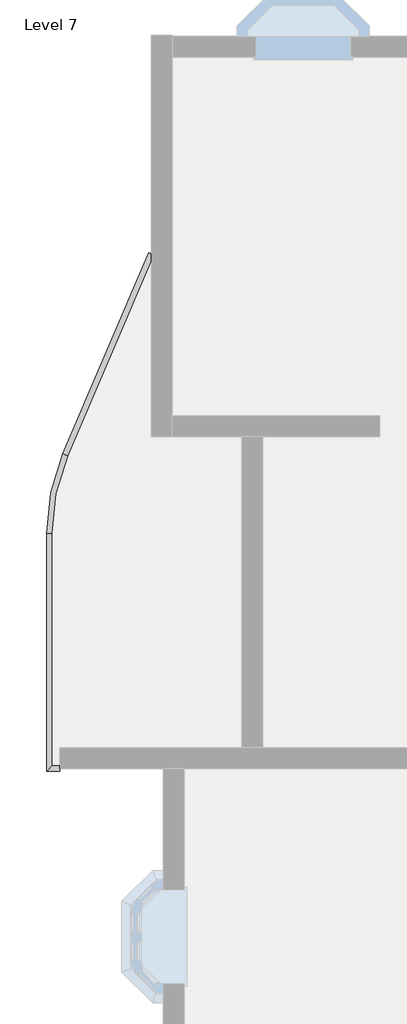
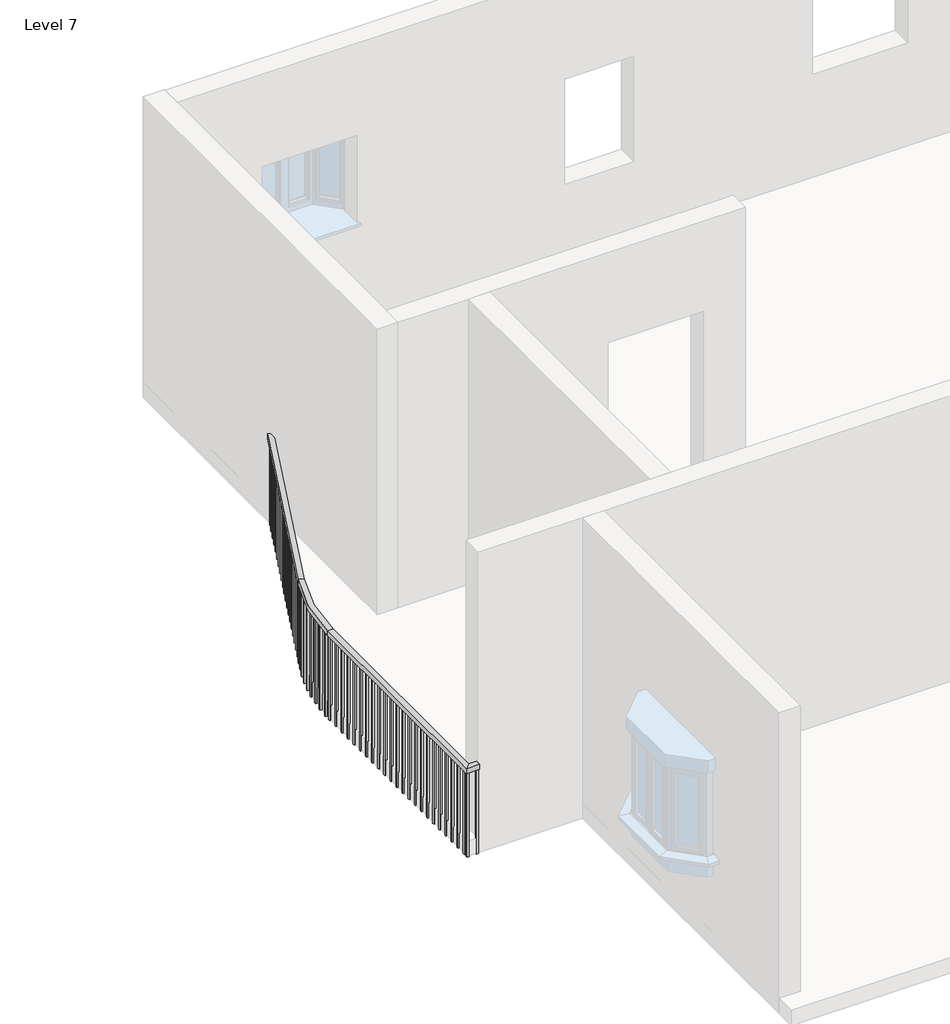
# One storey, part 7 of 14: 1 railing.
"""IFC4 building model written with IfcOpenShell, lengths in millimetres."""

from ifc_helpers import new_model, si_unit, frame, origin, place, context, project, spatial, polyline, circle_curve, outline, extrude, element, save
from ifc_brep_helpers import plane_surface, cylinder_surface, revolved_surface, advanced_brep

model = new_model("IFC4")

# Units and contexts
model_context = context("Model", 3, world=origin())
ifc_project = project(units=[si_unit("LENGTHUNIT", "METRE", prefix="MILLI")], contexts=[model_context])

# Site, building, storey
site = spatial("IfcSite", under=ifc_project)
building = spatial("IfcBuilding", under=site)
storey = spatial("IfcBuildingStorey", under=building, Name="Level 7", Elevation=18288.0)

# Railing
placement = place(None, origin())
element("IfcRailing", 1, ObjectType="Handrail - Rectangular", at=placement, inside=storey, context=model_context, shape_type="SolidModel", body=[
    advanced_brep(
    [(-12381.4379579, -2441.2590879, 19202.4), (-12381.4379579, -2441.2590879, 19151.6), (-12428.1364721, -2421.2618688, 19151.6), (-12428.1364721, -2421.2618688, 19202.4), (-13216.1814979, -4390.5942894, 19202.4), (-13216.1814979, -4390.5942894, 19151.6), (-13262.8800121, -4370.5970703, 19151.6), (-13262.8800121, -4370.5970703, 19202.4), (-13369.987215, -5140.4900045, 19151.6), (-13369.987215, -5140.4900045, 19202.4), (-13420.787215, -5140.4900045, 19151.6), (-13420.787215, -5140.4900045, 19202.4), (-13369.987215, -7396.5416506, 19202.4), (-13369.987215, -7396.5416506, 19151.6), (-13420.787215, -7447.3416506, 19151.6), (-13420.787215, -7447.3416506, 19202.4), (-13293.787215, -7396.5416506, 19202.4), (-13293.787215, -7447.3416506, 19202.4), (-13293.787215, -7447.3416506, 19151.6), (-13293.787215, -7396.5416506, 19151.6)],
    [
        (0, 1),
        (1, 2),
        (2, 3),
        (3, 0),
        (0, 4),
        (4, 5),
        (5, 1),
        (5, 6),
        (6, 2),
        (6, 7),
        (7, 3),
        (7, 4),
        (8, 5, circle_curve(frame((-11464.987215, -5140.4900045, 19151.6), z_axis=(0.0, 0.0, -1.0), x_axis=(-0.9192620907623801, 0.39364604467361003, 0.0)), 1905.0)),
        (4, 9, circle_curve(frame((-11464.987215, -5140.4900045, 19202.4), z_axis=(0.0, 0.0, 1.0), x_axis=(-0.9192620907623801, 0.39364604467361003, 0.0)), 1905.0)),
        (9, 8),
        (10, 6, circle_curve(frame((-11464.987215, -5140.4900045, 19151.6), z_axis=(0.0, 0.0, -1.0), x_axis=(-0.9192620907623801, 0.39364604467361003, 0.0)), 1955.8)),
        (8, 10),
        (11, 7, circle_curve(frame((-11464.987215, -5140.4900045, 19202.4), z_axis=(0.0, 0.0, -1.0), x_axis=(-0.9192620907623801, 0.39364604467361003, 0.0)), 1955.8)),
        (10, 11),
        (11, 9),
        (9, 12),
        (12, 13),
        (13, 8),
        (13, 14),
        (14, 10),
        (14, 15),
        (15, 11),
        (15, 12),
        (16, 17),
        (17, 18),
        (18, 19),
        (19, 16),
        (12, 16),
        (19, 13),
        (18, 14),
        (17, 15),
    ],
    [
        plane_surface(frame((-12404.787215, -2431.2604783, 19202.4), z_axis=(0.39364604467361003, 0.9192620907623801, 0.0), x_axis=(0.9192620907623801, -0.39364604467361003, 0.0))),
        plane_surface(frame((-12381.4379579, -2441.2590879, 19202.4), z_axis=(0.91926209076238, -0.39364604467361014, 0.0), x_axis=(-0.39364604467361014, -0.91926209076238, 0.0))),
        plane_surface(frame((-12381.4379579, -2441.2590879, 19151.6), z_axis=(0.0, 0.0, -1.0), x_axis=(-0.39364604467361014, -0.91926209076238, 0.0))),
        plane_surface(frame((-12428.1364721, -2421.2618688, 19151.6), z_axis=(-0.91926209076238, 0.39364604467361014, 0.0), x_axis=(-0.39364604467361014, -0.91926209076238, 0.0))),
        plane_surface(frame((-12428.1364721, -2421.2618688, 19202.4), z_axis=(0.0, 0.0, 1.0), x_axis=(-0.39364604467361014, -0.91926209076238, 0.0))),
        revolved_surface(polyline([(-13216.181497902333, -4390.594289396773, 19202.4), (-13216.181497902333, -4390.594289396773, 19151.6)]), (-11464.987215, -5140.4900045, 19202.4), (0.0, 0.0, 1.0)),
        plane_surface(frame((-11464.987215, -5140.4900045, 19151.6), z_axis=(0.0, 0.0, -1.0000000000000002), x_axis=(-0.9192620907623801, 0.39364604467361003, 0.0))),
        cylinder_surface(frame((-11464.987215, -5140.4900045, 19202.4), z_axis=(0.0, 0.0, 1.0), x_axis=(-0.9192620907623801, 0.39364604467361003, 0.0)), 1955.8),
        plane_surface(frame((-11464.987215, -5140.4900045, 19202.4), z_axis=(0.0, 0.0, 1.0000000000000002), x_axis=(-0.9192620907623801, 0.39364604467361003, 0.0))),
        plane_surface(frame((-13369.987215, -5140.4900045, 19202.4), z_axis=(1.0, 0.0, 0.0), x_axis=(0.0, -1.0, 0.0))),
        plane_surface(frame((-13369.987215, -5140.4900045, 19151.6), z_axis=(0.0, 0.0, -1.0), x_axis=(0.0, -1.0, 0.0))),
        plane_surface(frame((-13420.787215, -5140.4900045, 19151.6), z_axis=(-1.0, 0.0, 0.0), x_axis=(0.0, -1.0, 0.0))),
        plane_surface(frame((-13420.787215, -5140.4900045, 19202.4), z_axis=(0.0, 0.0, 1.0), x_axis=(0.0, -1.0, 0.0))),
        plane_surface(frame((-13293.787215, -7421.9416506, 19202.4), z_axis=(1.0, 0.0, 0.0), x_axis=(0.0, 1.0, 0.0))),
        plane_surface(frame((-13369.987215, -7396.5416506, 19202.4), z_axis=(0.0, 1.0, 0.0), x_axis=(1.0, 0.0, 0.0))),
        plane_surface(frame((-13369.987215, -7396.5416506, 19151.6), z_axis=(0.0, 0.0, -1.0), x_axis=(1.0, 0.0, 0.0))),
        plane_surface(frame((-13420.787215, -7447.3416506, 19151.6), z_axis=(0.0, -1.0, 0.0), x_axis=(1.0, 0.0, 0.0))),
        plane_surface(frame((-13420.787215, -7447.3416506, 19202.4), z_axis=(0.0, 0.0, 1.0), x_axis=(1.0, 0.0, 0.0))),
    ],
    [
        (0, [[1, 2, 3, 4]]),
        (1, [[-1, 5, 6, 7]]),
        (2, [[-2, -7, 8, 9]]),
        (3, [[-3, -9, 10, 11]]),
        (4, [[-4, -11, 12, -5]]),
        (5, [[13, -6, 14, 15]]),
        (6, [[16, -8, -13, 17]]),
        (7, [[18, -10, -16, 19]]),
        (8, [[-14, -12, -18, 20]]),
        (9, [[-15, 21, 22, 23]]),
        (10, [[-17, -23, 24, 25]]),
        (11, [[-19, -25, 26, 27]]),
        (12, [[-20, -27, 28, -21]]),
        (13, [[29, 30, 31, 32]]),
        (14, [[-22, 33, -32, 34]]),
        (15, [[-24, -34, -31, 35]]),
        (16, [[-26, -35, -30, 36]]),
        (17, [[-28, -36, -29, -33]]),
    ],
),
    extrude(outline(polyline([(-13404.912215, -7366.1650045), (-13385.862215, -7366.1650045), (-13385.862215, -7385.2150045), (-13404.912215, -7385.2150045), (-13404.912215, -7366.1650045)])), frame((0.0, 0.0, 18288.0), z_axis=(0.0, 0.0, 1.0), x_axis=(1.0, 0.0, 0.0)), (0.0, 0.0, 1.0), 863.6),
    extrude(outline(polyline([(-13404.912215, -7264.5650045), (-13385.862215, -7264.5650045), (-13385.862215, -7283.6150045), (-13404.912215, -7283.6150045), (-13404.912215, -7264.5650045)])), frame((0.0, 0.0, 18288.0), z_axis=(0.0, 0.0, 1.0), x_axis=(1.0, 0.0, 0.0)), (0.0, 0.0, 1.0), 863.6),
    extrude(outline(polyline([(-13404.912215, -7162.9650045), (-13385.862215, -7162.9650045), (-13385.862215, -7182.0150045), (-13404.912215, -7182.0150045), (-13404.912215, -7162.9650045)])), frame((0.0, 0.0, 18288.0), z_axis=(0.0, 0.0, 1.0), x_axis=(1.0, 0.0, 0.0)), (0.0, 0.0, 1.0), 863.6),
    extrude(outline(polyline([(-13404.912215, -7061.3650045), (-13385.862215, -7061.3650045), (-13385.862215, -7080.4150045), (-13404.912215, -7080.4150045), (-13404.912215, -7061.3650045)])), frame((0.0, 0.0, 18288.0), z_axis=(0.0, 0.0, 1.0), x_axis=(1.0, 0.0, 0.0)), (0.0, 0.0, 1.0), 863.6),
    extrude(outline(polyline([(-13404.912215, -6959.7650045), (-13385.862215, -6959.7650045), (-13385.862215, -6978.8150045), (-13404.912215, -6978.8150045), (-13404.912215, -6959.7650045)])), frame((0.0, 0.0, 18288.0), z_axis=(0.0, 0.0, 1.0), x_axis=(1.0, 0.0, 0.0)), (0.0, 0.0, 1.0), 863.6),
    extrude(outline(polyline([(-13404.912215, -6858.1650045), (-13385.862215, -6858.1650045), (-13385.862215, -6877.2150045), (-13404.912215, -6877.2150045), (-13404.912215, -6858.1650045)])), frame((0.0, 0.0, 18288.0), z_axis=(0.0, 0.0, 1.0), x_axis=(1.0, 0.0, 0.0)), (0.0, 0.0, 1.0), 863.6),
    extrude(outline(polyline([(-13404.912215, -6756.5650045), (-13385.862215, -6756.5650045), (-13385.862215, -6775.6150045), (-13404.912215, -6775.6150045), (-13404.912215, -6756.5650045)])), frame((0.0, 0.0, 18288.0), z_axis=(0.0, 0.0, 1.0), x_axis=(1.0, 0.0, 0.0)), (0.0, 0.0, 1.0), 863.6),
    extrude(outline(polyline([(-13404.912215, -6654.9650045), (-13385.862215, -6654.9650045), (-13385.862215, -6674.0150045), (-13404.912215, -6674.0150045), (-13404.912215, -6654.9650045)])), frame((0.0, 0.0, 18288.0), z_axis=(0.0, 0.0, 1.0), x_axis=(1.0, 0.0, 0.0)), (0.0, 0.0, 1.0), 863.6),
    extrude(outline(polyline([(-13404.912215, -6553.3650045), (-13385.862215, -6553.3650045), (-13385.862215, -6572.4150045), (-13404.912215, -6572.4150045), (-13404.912215, -6553.3650045)])), frame((0.0, 0.0, 18288.0), z_axis=(0.0, 0.0, 1.0), x_axis=(1.0, 0.0, 0.0)), (0.0, 0.0, 1.0), 863.6),
    extrude(outline(polyline([(-13404.912215, -6451.7650045), (-13385.862215, -6451.7650045), (-13385.862215, -6470.8150045), (-13404.912215, -6470.8150045), (-13404.912215, -6451.7650045)])), frame((0.0, 0.0, 18288.0), z_axis=(0.0, 0.0, 1.0), x_axis=(1.0, 0.0, 0.0)), (0.0, 0.0, 1.0), 863.6),
    extrude(outline(polyline([(-13404.912215, -6350.1650045), (-13385.862215, -6350.1650045), (-13385.862215, -6369.2150045), (-13404.912215, -6369.2150045), (-13404.912215, -6350.1650045)])), frame((0.0, 0.0, 18288.0), z_axis=(0.0, 0.0, 1.0), x_axis=(1.0, 0.0, 0.0)), (0.0, 0.0, 1.0), 863.6),
    extrude(outline(polyline([(-13404.912215, -6248.5650045), (-13385.862215, -6248.5650045), (-13385.862215, -6267.6150045), (-13404.912215, -6267.6150045), (-13404.912215, -6248.5650045)])), frame((0.0, 0.0, 18288.0), z_axis=(0.0, 0.0, 1.0), x_axis=(1.0, 0.0, 0.0)), (0.0, 0.0, 1.0), 863.6),
    extrude(outline(polyline([(-13404.912215, -6146.9650045), (-13385.862215, -6146.9650045), (-13385.862215, -6166.0150045), (-13404.912215, -6166.0150045), (-13404.912215, -6146.9650045)])), frame((0.0, 0.0, 18288.0), z_axis=(0.0, 0.0, 1.0), x_axis=(1.0, 0.0, 0.0)), (0.0, 0.0, 1.0), 863.6),
    extrude(outline(polyline([(-13404.912215, -6045.3650045), (-13385.862215, -6045.3650045), (-13385.862215, -6064.4150045), (-13404.912215, -6064.4150045), (-13404.912215, -6045.3650045)])), frame((0.0, 0.0, 18288.0), z_axis=(0.0, 0.0, 1.0), x_axis=(1.0, 0.0, 0.0)), (0.0, 0.0, 1.0), 863.6),
    extrude(outline(polyline([(-13404.912215, -5943.7650045), (-13385.862215, -5943.7650045), (-13385.862215, -5962.8150045), (-13404.912215, -5962.8150045), (-13404.912215, -5943.7650045)])), frame((0.0, 0.0, 18288.0), z_axis=(0.0, 0.0, 1.0), x_axis=(1.0, 0.0, 0.0)), (0.0, 0.0, 1.0), 863.6),
    extrude(outline(polyline([(-13404.912215, -5842.1650045), (-13385.862215, -5842.1650045), (-13385.862215, -5861.2150045), (-13404.912215, -5861.2150045), (-13404.912215, -5842.1650045)])), frame((0.0, 0.0, 18288.0), z_axis=(0.0, 0.0, 1.0), x_axis=(1.0, 0.0, 0.0)), (0.0, 0.0, 1.0), 863.6),
    extrude(outline(polyline([(-13404.912215, -5740.5650045), (-13385.862215, -5740.5650045), (-13385.862215, -5759.6150045), (-13404.912215, -5759.6150045), (-13404.912215, -5740.5650045)])), frame((0.0, 0.0, 18288.0), z_axis=(0.0, 0.0, 1.0), x_axis=(1.0, 0.0, 0.0)), (0.0, 0.0, 1.0), 863.6),
    extrude(outline(polyline([(-13404.912215, -5638.9650045), (-13385.862215, -5638.9650045), (-13385.862215, -5658.0150045), (-13404.912215, -5658.0150045), (-13404.912215, -5638.9650045)])), frame((0.0, 0.0, 18288.0), z_axis=(0.0, 0.0, 1.0), x_axis=(1.0, 0.0, 0.0)), (0.0, 0.0, 1.0), 863.6),
    extrude(outline(polyline([(-13404.912215, -5537.3650045), (-13385.862215, -5537.3650045), (-13385.862215, -5556.4150045), (-13404.912215, -5556.4150045), (-13404.912215, -5537.3650045)])), frame((0.0, 0.0, 18288.0), z_axis=(0.0, 0.0, 1.0), x_axis=(1.0, 0.0, 0.0)), (0.0, 0.0, 1.0), 863.6),
    extrude(outline(polyline([(-13404.912215, -5435.7650045), (-13385.862215, -5435.7650045), (-13385.862215, -5454.8150045), (-13404.912215, -5454.8150045), (-13404.912215, -5435.7650045)])), frame((0.0, 0.0, 18288.0), z_axis=(0.0, 0.0, 1.0), x_axis=(1.0, 0.0, 0.0)), (0.0, 0.0, 1.0), 863.6),
    extrude(outline(polyline([(-13404.912215, -5334.1650045), (-13385.862215, -5334.1650045), (-13385.862215, -5353.2150045), (-13404.912215, -5353.2150045), (-13404.912215, -5334.1650045)])), frame((0.0, 0.0, 18288.0), z_axis=(0.0, 0.0, 1.0), x_axis=(1.0, 0.0, 0.0)), (0.0, 0.0, 1.0), 863.6),
    extrude(outline(polyline([(-13404.912215, -5232.5650045), (-13385.862215, -5232.5650045), (-13385.862215, -5251.6150045), (-13404.912215, -5251.6150045), (-13404.912215, -5232.5650045)])), frame((0.0, 0.0, 18288.0), z_axis=(0.0, 0.0, 1.0), x_axis=(1.0, 0.0, 0.0)), (0.0, 0.0, 1.0), 863.6),
    extrude(outline(polyline([(-13403.2986616, -5060.8127369), (-13384.2611239, -5061.5016911), (-13384.9500781, -5080.5392288), (-13403.9876158, -5079.8502746), (-13403.2986616, -5060.8127369)])), frame((0.0, 0.0, 18288.0), z_axis=(0.0, 0.0, 1.0), x_axis=(1.0, 0.0, 0.0)), (0.0, 0.0, 1.0), 863.6),
    extrude(outline(polyline([(-13396.4230348, -4958.9537683), (-13377.4481028, -4960.6432816), (-13379.1376161, -4979.6182136), (-13398.1125481, -4977.9287003), (-13396.4230348, -4958.9537683)])), frame((0.0, 0.0, 18288.0), z_axis=(0.0, 0.0, 1.0), x_axis=(1.0, 0.0, 0.0)), (0.0, 0.0, 1.0), 863.6),
    extrude(outline(polyline([(-13384.1984052, -4857.5975541), (-13365.3386289, -4860.2829475), (-13368.0240223, -4879.1427238), (-13386.8837986, -4876.4573304), (-13384.1984052, -4857.5975541)])), frame((0.0, 0.0, 18288.0), z_axis=(0.0, 0.0, 1.0), x_axis=(1.0, 0.0, 0.0)), (0.0, 0.0, 1.0), 863.6),
    extrude(outline(polyline([(-13366.6586282, -4757.0247946), (-13347.9662387, -4760.698631), (-13351.6400752, -4779.3910205), (-13370.3324647, -4775.7171841), (-13366.6586282, -4757.0247946)])), frame((0.0, 0.0, 18288.0), z_axis=(0.0, 0.0, 1.0), x_axis=(1.0, 0.0, 0.0)), (0.0, 0.0, 1.0), 863.6),
    extrude(outline(polyline([(-13343.8522793, -4657.5140204), (-13325.3790441, -4662.1661254), (-13330.0311492, -4680.6393606), (-13348.5043844, -4675.9872556), (-13343.8522793, -4657.5140204)])), frame((0.0, 0.0, 18288.0), z_axis=(0.0, 0.0, 1.0), x_axis=(1.0, 0.0, 0.0)), (0.0, 0.0, 1.0), 863.6),
    extrude(outline(polyline([(-13315.8425193, -4559.340821), (-13297.6395991, -4564.9583109), (-13303.257089, -4583.1612312), (-13321.4600093, -4577.5437413), (-13315.8425193, -4559.340821)])), frame((0.0, 0.0, 18288.0), z_axis=(0.0, 0.0, 1.0), x_axis=(1.0, 0.0, 0.0)), (0.0, 0.0, 1.0), 863.6),
    extrude(outline(polyline([(-13282.7069198, -4462.7770815), (-13264.8247264, -4469.344399), (-13271.3920438, -4487.2265924), (-13289.2742372, -4480.659275), (-13282.7069198, -4462.7770815)])), frame((0.0, 0.0, 18288.0), z_axis=(0.0, 0.0, 1.0), x_axis=(1.0, 0.0, 0.0)), (0.0, 0.0, 1.0), 863.6),
    extrude(outline(polyline([(-13209.6824706, -4286.6955968), (-13192.1705278, -4294.1945539), (-13199.6694849, -4311.7064967), (-13217.1814277, -4304.2075396), (-13209.6824706, -4286.6955968)])), frame((0.0, 0.0, 18288.0), z_axis=(0.0, 0.0, 1.0), x_axis=(1.0, 0.0, 0.0)), (0.0, 0.0, 1.0), 863.6),
    extrude(outline(polyline([(-13169.6880325, -4193.2985683), (-13152.1760896, -4200.7975255), (-13159.6750468, -4218.3094683), (-13177.1869896, -4210.8105112), (-13169.6880325, -4193.2985683)])), frame((0.0, 0.0, 18288.0), z_axis=(0.0, 0.0, 1.0), x_axis=(1.0, 0.0, 0.0)), (0.0, 0.0, 1.0), 863.6),
    extrude(outline(polyline([(-13129.6935943, -4099.9015399), (-13112.1816515, -4107.4004971), (-13119.6806086, -4124.9124399), (-13137.1925515, -4117.4134827), (-13129.6935943, -4099.9015399)])), frame((0.0, 0.0, 18288.0), z_axis=(0.0, 0.0, 1.0), x_axis=(1.0, 0.0, 0.0)), (0.0, 0.0, 1.0), 863.6),
    extrude(outline(polyline([(-13089.6991562, -4006.5045115), (-13072.1872133, -4014.0034686), (-13079.6861705, -4031.5154115), (-13097.1981133, -4024.0164543), (-13089.6991562, -4006.5045115)])), frame((0.0, 0.0, 18288.0), z_axis=(0.0, 0.0, 1.0), x_axis=(1.0, 0.0, 0.0)), (0.0, 0.0, 1.0), 863.6),
    extrude(outline(polyline([(-13049.704718, -3913.1074831), (-13032.1927752, -3920.6064402), (-13039.6917324, -3938.1183831), (-13057.2036752, -3930.6194259), (-13049.704718, -3913.1074831)])), frame((0.0, 0.0, 18288.0), z_axis=(0.0, 0.0, 1.0), x_axis=(1.0, 0.0, 0.0)), (0.0, 0.0, 1.0), 863.6),
    extrude(outline(polyline([(-13009.7102799, -3819.7104546), (-12992.1983371, -3827.2094118), (-12999.6972942, -3844.7213546), (-13017.209237, -3837.2223975), (-13009.7102799, -3819.7104546)])), frame((0.0, 0.0, 18288.0), z_axis=(0.0, 0.0, 1.0), x_axis=(1.0, 0.0, 0.0)), (0.0, 0.0, 1.0), 863.6),
    extrude(outline(polyline([(-12969.7158418, -3726.3134262), (-12952.2038989, -3733.8123834), (-12959.7028561, -3751.3243262), (-12977.2147989, -3743.8253691), (-12969.7158418, -3726.3134262)])), frame((0.0, 0.0, 18288.0), z_axis=(0.0, 0.0, 1.0), x_axis=(1.0, 0.0, 0.0)), (0.0, 0.0, 1.0), 863.6),
    extrude(outline(polyline([(-12929.7214036, -3632.9163978), (-12912.2094608, -3640.415355), (-12919.7084179, -3657.9272978), (-12937.2203608, -3650.4283406), (-12929.7214036, -3632.9163978)])), frame((0.0, 0.0, 18288.0), z_axis=(0.0, 0.0, 1.0), x_axis=(1.0, 0.0, 0.0)), (0.0, 0.0, 1.0), 863.6),
    extrude(outline(polyline([(-12889.7269655, -3539.5193694), (-12872.2150227, -3547.0183265), (-12879.7139798, -3564.5302694), (-12897.2259226, -3557.0313122), (-12889.7269655, -3539.5193694)])), frame((0.0, 0.0, 18288.0), z_axis=(0.0, 0.0, 1.0), x_axis=(1.0, 0.0, 0.0)), (0.0, 0.0, 1.0), 863.6),
    extrude(outline(polyline([(-12849.7325273, -3446.122341), (-12832.2205845, -3453.6212981), (-12839.7195417, -3471.1332409), (-12857.2314845, -3463.6342838), (-12849.7325273, -3446.122341)])), frame((0.0, 0.0, 18288.0), z_axis=(0.0, 0.0, 1.0), x_axis=(1.0, 0.0, 0.0)), (0.0, 0.0, 1.0), 863.6),
    extrude(outline(polyline([(-12809.7380892, -3352.7253125), (-12792.2261464, -3360.2242697), (-12799.7251035, -3377.7362125), (-12817.2370464, -3370.2372554), (-12809.7380892, -3352.7253125)])), frame((0.0, 0.0, 18288.0), z_axis=(0.0, 0.0, 1.0), x_axis=(1.0, 0.0, 0.0)), (0.0, 0.0, 1.0), 863.6),
    extrude(outline(polyline([(-12769.7436511, -3259.3282841), (-12752.2317082, -3266.8272413), (-12759.7306654, -3284.3391841), (-12777.2426082, -3276.8402269), (-12769.7436511, -3259.3282841)])), frame((0.0, 0.0, 18288.0), z_axis=(0.0, 0.0, 1.0), x_axis=(1.0, 0.0, 0.0)), (0.0, 0.0, 1.0), 863.6),
    extrude(outline(polyline([(-12729.7492129, -3165.9312557), (-12712.2372701, -3173.4302129), (-12719.7362272, -3190.9421557), (-12737.2481701, -3183.4431985), (-12729.7492129, -3165.9312557)])), frame((0.0, 0.0, 18288.0), z_axis=(0.0, 0.0, 1.0), x_axis=(1.0, 0.0, 0.0)), (0.0, 0.0, 1.0), 863.6),
    extrude(outline(polyline([(-12689.7547748, -3072.5342273), (-12672.242832, -3080.0331844), (-12679.7417891, -3097.5451273), (-12697.2537319, -3090.0461701), (-12689.7547748, -3072.5342273)])), frame((0.0, 0.0, 18288.0), z_axis=(0.0, 0.0, 1.0), x_axis=(1.0, 0.0, 0.0)), (0.0, 0.0, 1.0), 863.6),
    extrude(outline(polyline([(-12649.7603366, -2979.1371989), (-12632.2483938, -2986.636156), (-12639.747351, -3004.1480988), (-12657.2592938, -2996.6491417), (-12649.7603366, -2979.1371989)])), frame((0.0, 0.0, 18288.0), z_axis=(0.0, 0.0, 1.0), x_axis=(1.0, 0.0, 0.0)), (0.0, 0.0, 1.0), 863.6),
    extrude(outline(polyline([(-12609.7658985, -2885.7401704), (-12592.2539557, -2893.2391276), (-12599.7529128, -2910.7510704), (-12617.2648557, -2903.2521133), (-12609.7658985, -2885.7401704)])), frame((0.0, 0.0, 18288.0), z_axis=(0.0, 0.0, 1.0), x_axis=(1.0, 0.0, 0.0)), (0.0, 0.0, 1.0), 863.6),
    extrude(outline(polyline([(-12569.7714604, -2792.343142), (-12552.2595175, -2799.8420992), (-12559.7584747, -2817.354042), (-12577.2704175, -2809.8550848), (-12569.7714604, -2792.343142)])), frame((0.0, 0.0, 18288.0), z_axis=(0.0, 0.0, 1.0), x_axis=(1.0, 0.0, 0.0)), (0.0, 0.0, 1.0), 863.6),
    extrude(outline(polyline([(-12529.7770222, -2698.9461136), (-12512.2650794, -2706.4450707), (-12519.7640366, -2723.9570136), (-12537.2759794, -2716.4580564), (-12529.7770222, -2698.9461136)])), frame((0.0, 0.0, 18288.0), z_axis=(0.0, 0.0, 1.0), x_axis=(1.0, 0.0, 0.0)), (0.0, 0.0, 1.0), 863.6),
    extrude(outline(polyline([(-12489.7825841, -2605.5490852), (-12472.2706413, -2613.0480423), (-12479.7695984, -2630.5599852), (-12497.2815412, -2623.061028), (-12489.7825841, -2605.5490852)])), frame((0.0, 0.0, 18288.0), z_axis=(0.0, 0.0, 1.0), x_axis=(1.0, 0.0, 0.0)), (0.0, 0.0, 1.0), 863.6),
    extrude(outline(polyline([(-12449.788146, -2512.1520567), (-12432.2762031, -2519.6510139), (-12439.7751603, -2537.1629567), (-12457.2871031, -2529.6639996), (-12449.788146, -2512.1520567)])), frame((0.0, 0.0, 18288.0), z_axis=(0.0, 0.0, 1.0), x_axis=(1.0, 0.0, 0.0)), (0.0, 0.0, 1.0), 863.6),
    extrude(outline(polyline([(-13404.912215, -7412.4166506), (-13385.862215, -7412.4166506), (-13385.862215, -7431.4666506), (-13404.912215, -7431.4666506), (-13404.912215, -7412.4166506)])), frame((0.0, 0.0, 18288.0), z_axis=(0.0, 0.0, 1.0), x_axis=(1.0, 0.0, 0.0)), (0.0, 0.0, 1.0), 863.6),
    extrude(outline(polyline([(-13404.912215, -5130.9650045), (-13385.862215, -5130.9650045), (-13385.862215, -5150.0150045), (-13404.912215, -5150.0150045), (-13404.912215, -5130.9650045)])), frame((0.0, 0.0, 18288.0), z_axis=(0.0, 0.0, 1.0), x_axis=(1.0, 0.0, 0.0)), (0.0, 0.0, 1.0), 863.6),
    extrude(outline(polyline([(-13244.5372478, -4368.0902299), (-13227.025305, -4375.589187), (-13234.5242621, -4393.1011299), (-13252.036205, -4385.6021727), (-13244.5372478, -4368.0902299)])), frame((0.0, 0.0, 18288.0), z_axis=(0.0, 0.0, 1.0), x_axis=(1.0, 0.0, 0.0)), (0.0, 0.0, 1.0), 863.6),
    extrude(outline(polyline([(-13312.837215, -7431.4666506), (-13312.837215, -7412.4166506), (-13293.787215, -7412.4166506), (-13293.787215, -7431.4666506), (-13312.837215, -7431.4666506)])), frame((0.0, 0.0, 18288.0), z_axis=(0.0, 0.0, 1.0), x_axis=(1.0, 0.0, 0.0)), (0.0, 0.0, 1.0), 863.6),
    extrude(outline(polyline([(-12413.5431864, -2427.5109997), (-12396.0312436, -2435.0099569), (-12403.5302007, -2452.5218997), (-12421.0421435, -2445.0229426), (-12413.5431864, -2427.5109997)])), frame((0.0, 0.0, 18288.0), z_axis=(0.0, 0.0, 1.0), x_axis=(1.0, 0.0, 0.0)), (0.0, 0.0, 1.0), 863.6),
])

save(model, "model.ifc")

# Revit data of these elements
# Type "Handrail - Rectangular"
#   Assembly Code = "C2010400"
#   built-in parameter 1008612 = 0.0416667 (stored number, unit not read)
#   built-in parameter 1008611 = 0.0416667 (stored number, unit not read)
#   built-in parameter 1008609 = 0.333333 (stored number, unit not read)
#   built-in parameter 1008604 = 0.166667 (stored number, unit not read)
#   built-in parameter 1008603 = 0.166667 (stored number, unit not read)
#   Railing Height = 3' - 0"
#   built-in parameter 1008630 = 2
#   built-in parameter 1008610 = 2
#   built-in parameter 1008618 = Baluster - Square : 3/4"
# Element 1 (IfcRailing, "Handrail - Rectangular")
#   Phase Created = New Construction
